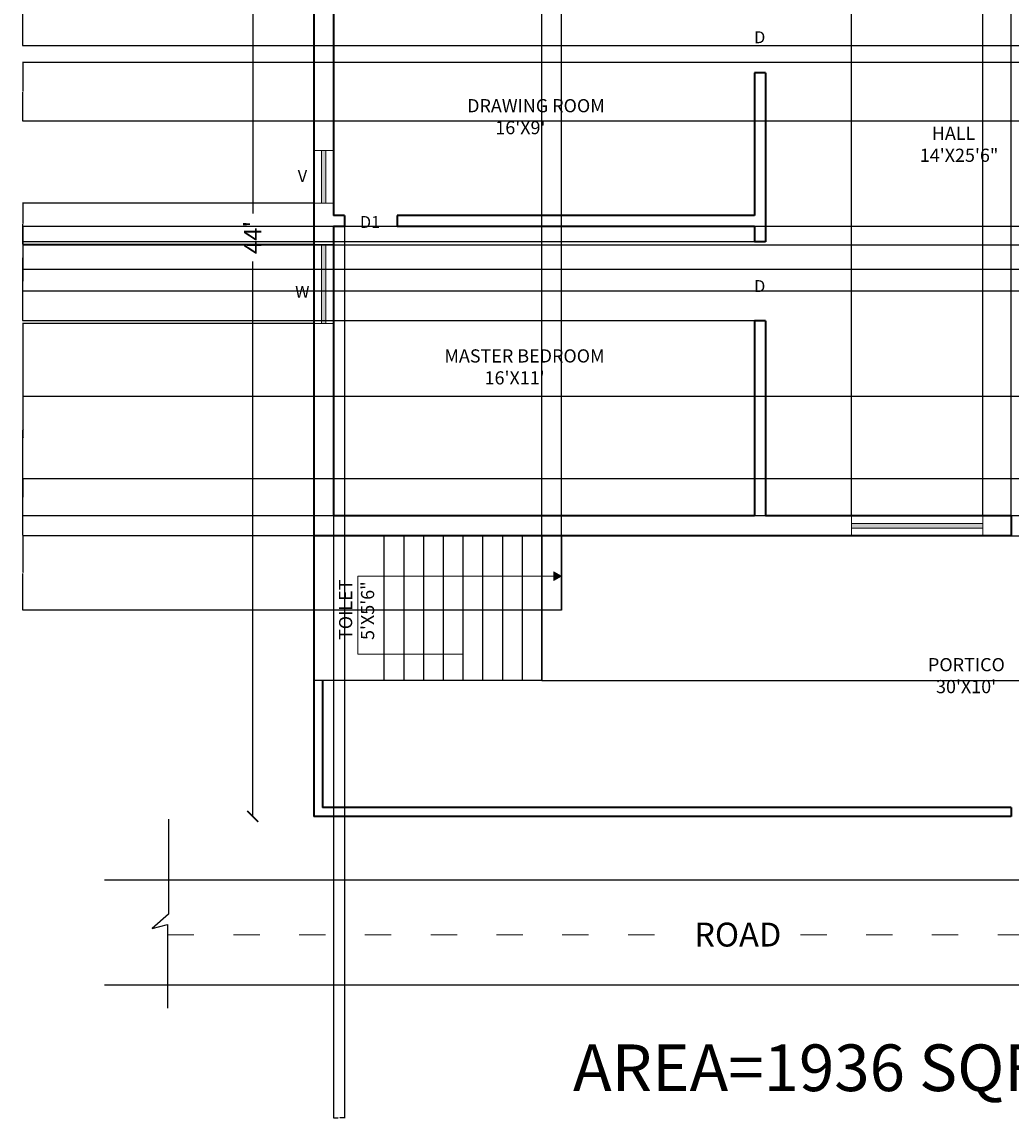
# Model space of a CAD drawing. Units: inches. Extents: x 320 to 1055, y -655 to 96.
# Tile 1 of 4: x 320 to 771, y -655 to -155. Entities that reach past the tile are written whole.
import ezdxf

# ---------------------------------------------------------------- set-up
doc = ezdxf.new("R2010")
doc.units = ezdxf.units.IN
doc.header["$MEASUREMENT"] = 0
doc.linetypes.add('ACAD_ISO03W100', pattern=[30, 12, -18])
for name, color, linetype, lineweight in [('A-ANNO-DIMS', 2, 'Continuous', 18), ('A-ANNO-IDEN', 1, 'Continuous', 18), ('A-ANNO-SYMB', 1, 'Continuous', 18), ('A-ANNO-TEXT', 8, 'Continuous', 18), ('A-AREA-IDEN', 8, 'Continuous', 18), ('A-FLOR-STRS', 1, 'Continuous', 25), ('A-GLAZ-PATT', 5, 'Continuous', 13), ('C-ROAD', 1, 'Continuous', 25), ('C-ROAD-CNTR', 1, 'ACAD_ISO03W100', 18), ('wall', 1, 'Continuous', 35), ('win', 5, 'Continuous', 18)]:
    doc.layers.add(name, color=color, linetype=linetype, lineweight=lineweight)
doc.styles.get("Standard").update_dxf_attribs({"font": 'arial.ttf'})
doc.dimstyles.get("Standard").update_dxf_attribs({"dimtxt": 0.18, "dimasz": 0.18, "dimexe": 0.18, "dimexo": 0.0625, "dimgap": 0.09, "dimtad": 0, "dimtih": 1, "dimtoh": 1, "dimdec": 1, "dimzin": 0, "dimdsep": 46, "dimlunit": 4, "dimtxsty": 'Standard', "dimcen": 0.09, "dimadec": 0, "dimazin": 0, "dimtfac": 1, "dimtdec": 1, "dimtofl": 0, "dimtmove": 0, "dimatfit": 3, "dimfxl": 1, "dimtolj": 1, "dimtzin": 0, "dimarcsym": 0})

# ---------------------------------------------------------------- blocks, each defined once
blk = doc.blocks.new('_ArchTick')
at = {"color": 0, "linetype": 'ByBlock', "const_width": 0.15}
blk.add_lwpolyline([(-0.5, -0.5), (0.5, 0.5)], dxfattribs=at)
blk = doc.blocks.new('*D2')
at = {"layer": 'A-ANNO-DIMS', "color": 0, "lineweight": -2, "transparency": 16777216}
for p, q in [((425, 10.26), (425, -242.79)), ((425, -517.74), (425, -264.69))]:
    blk.add_line(p, q, dxfattribs=at)
at = {"layer": 'Defpoints', "color": 0, "transparency": 16777216}
for p in [(452.86, 10.26), (425, -517.74), (452.86, -517.74)]:
    blk.add_point(p, dxfattribs=at)
at = {"layer": 'A-ANNO-DIMS', "color": 0, "lineweight": -2, "transparency": 16777216, "xscale": 5, "yscale": 5, "zscale": 5}
for p, rotation in [((425, 10.26), 90), ((425, -517.74), 270)]:
    blk.add_blockref('_ArchTick', p, dxfattribs=dict(at, rotation=rotation))
at = {"layer": 'A-ANNO-DIMS', "color": 0, "transparency": 16777216, "insert": (425, -253.74), "char_height": 8, "attachment_point": 5, "rotation": 90}
blk.add_mtext("\\A1;44'", dxfattribs=at)
blk = doc.blocks.new('WINDOW-36IN')
for p, q in [((0, 36), (9, 36)), ((3.5, 36), (3.5, 0)), ((5.5, 36), (5.5, 0)), ((0, 0), (9, 0))]:
    blk.add_line(p, q)
blk = doc.blocks.new('VENT-24IN')
for p, q in [((0, 0), (0, 9)), ((0, 5.5), (24, 5.5)), ((24, 0), (24, 9)), ((0, 3.5), (24, 3.5))]:
    blk.add_line(p, q)
blk = doc.blocks.new('*D21')
at = {"layer": 'A-ANNO-DIMS', "color": 0, "lineweight": -2, "transparency": 16777216}
for p, q in [((698.05, -380.67), (698.05, 47.57)), ((698.23, 47.39), (727.72, 47.39)), ((757.87, 47.39), (728.38, 47.39)), ((758.05, -380.67), (758.05, 47.57))]:
    blk.add_line(p, q, dxfattribs=at)
at = {"layer": 'A-ANNO-DIMS', "color": 0, "transparency": 16777216}
for points in [[(698.23, 47.42), (698.23, 47.36), (698.05, 47.39)], [(757.87, 47.42), (757.87, 47.36), (758.05, 47.39)]]:
    blk.add_solid(points, dxfattribs=at)
at = {"layer": 'Defpoints', "color": 0, "transparency": 16777216}
for p in [(758.05, 47.39), (698.05, -380.74), (758.05, -380.74)]:
    blk.add_point(p, dxfattribs=at)
at = {"layer": 'A-ANNO-DIMS', "color": 0, "transparency": 16777216, "insert": (728.05, 47.39), "char_height": 0.18, "attachment_point": 5}
blk.add_mtext('\\A1;5\'-0"', dxfattribs=at)
blk = doc.blocks.new('*D22')
at = {"layer": 'A-ANNO-DIMS', "color": 0, "lineweight": -2, "transparency": 16777216}
for p, q in [((658.8, -255.74), (320.04, -255.74)), ((320.22, -255.92), (320.22, -273.55)), ((320.22, -291.56), (320.22, -273.92)), ((658.8, -291.74), (320.04, -291.74))]:
    blk.add_line(p, q, dxfattribs=at)
at = {"layer": 'A-ANNO-DIMS', "color": 0, "transparency": 16777216}
for points in [[(320.19, -255.92), (320.25, -255.92), (320.22, -255.74)], [(320.19, -291.56), (320.25, -291.56), (320.22, -291.74)]]:
    blk.add_solid(points, dxfattribs=at)
at = {"layer": 'Defpoints', "color": 0, "transparency": 16777216}
for p in [(658.86, -255.74), (320.22, -291.74), (658.86, -291.74)]:
    blk.add_point(p, dxfattribs=at)
at = {"layer": 'A-ANNO-DIMS', "color": 0, "transparency": 16777216, "insert": (320.22, -273.74), "char_height": 0.18, "attachment_point": 5}
blk.add_mtext('\\A1;3\'-0"', dxfattribs=at)
blk = doc.blocks.new('*D26')
at = {"layer": 'A-ANNO-DIMS', "color": 0, "lineweight": -2, "transparency": 16777216}
for p, q in [((941.8, -248.74), (320.04, -248.74)), ((320.22, -248.92), (320.22, -263.27)), ((320.22, -278), (320.22, -263.64)), ((941.8, -278.18), (320.04, -278.18))]:
    blk.add_line(p, q, dxfattribs=at)
at = {"layer": 'A-ANNO-DIMS', "color": 0, "transparency": 16777216}
for points in [[(320.19, -248.92), (320.25, -248.92), (320.22, -248.74)], [(320.19, -278), (320.25, -278), (320.22, -278.18)]]:
    blk.add_solid(points, dxfattribs=at)
at = {"layer": 'Defpoints', "color": 0, "transparency": 16777216}
for p in [(941.86, -248.74), (320.22, -278.18), (941.86, -278.18)]:
    blk.add_point(p, dxfattribs=at)
at = {"layer": 'A-ANNO-DIMS', "color": 0, "transparency": 16777216, "insert": (320.22, -263.46), "char_height": 0.18, "attachment_point": 5}
blk.add_mtext('\\A1;2\'-5 1/2"', dxfattribs=at)
blk = doc.blocks.new('*D27')
at = {"layer": 'A-ANNO-DIMS', "color": 0, "lineweight": -2, "transparency": 16777216}
for p, q in [((943.8, -326.24), (320.04, -326.24)), ((320.22, -326.42), (320.22, -344.83)), ((320.22, -363.61), (320.22, -345.2)), ((943.8, -363.79), (320.04, -363.79))]:
    blk.add_line(p, q, dxfattribs=at)
at = {"layer": 'A-ANNO-DIMS', "color": 0, "transparency": 16777216}
for points in [[(320.19, -326.42), (320.25, -326.42), (320.22, -326.24)], [(320.19, -363.61), (320.25, -363.61), (320.22, -363.79)]]:
    blk.add_solid(points, dxfattribs=at)
at = {"layer": 'Defpoints', "color": 0, "transparency": 16777216}
for p in [(943.86, -326.24), (320.22, -363.79), (943.86, -363.79)]:
    blk.add_point(p, dxfattribs=at)
at = {"layer": 'A-ANNO-DIMS', "color": 0, "transparency": 16777216, "insert": (320.22, -345.02), "char_height": 0.18, "attachment_point": 5}
blk.add_mtext('\\A1;3\'-1 1/2"', dxfattribs=at)
blk = doc.blocks.new('*D32')
at = {"layer": 'A-ANNO-DIMS', "color": 0, "lineweight": -2, "transparency": 16777216}
for p, q in [((883.46, -174.02), (320.04, -174.02)), ((320.22, -174.2), (320.22, -187.17)), ((320.22, -200.52), (320.22, -187.54)), ((883.46, -200.7), (320.04, -200.7))]:
    blk.add_line(p, q, dxfattribs=at)
at = {"layer": 'A-ANNO-DIMS', "color": 0, "transparency": 16777216}
for points in [[(320.19, -174.2), (320.25, -174.2), (320.22, -174.02)], [(320.19, -200.52), (320.25, -200.52), (320.22, -200.7)]]:
    blk.add_solid(points, dxfattribs=at)
at = {"layer": 'Defpoints', "color": 0, "transparency": 16777216}
for p in [(883.52, -174.02), (320.22, -200.7), (883.52, -200.7)]:
    blk.add_point(p, dxfattribs=at)
at = {"layer": 'A-ANNO-DIMS', "color": 0, "transparency": 16777216, "insert": (320.22, -187.36), "char_height": 0.18, "attachment_point": 5}
blk.add_mtext('\\A1;2\'-2 1/2"', dxfattribs=at)
blk = doc.blocks.new('*D33')
at = {"layer": 'A-ANNO-DIMS', "color": 0, "lineweight": -2, "transparency": 16777216}
for p, q in [((452.86, -389.67), (452.86, 47.57)), ((453.04, 47.39), (509.03, 47.39)), ((565.68, 47.39), (509.69, 47.39)), ((565.86, -389.67), (565.86, 47.57))]:
    blk.add_line(p, q, dxfattribs=at)
at = {"layer": 'A-ANNO-DIMS', "color": 0, "transparency": 16777216}
for points in [[(453.04, 47.42), (453.04, 47.36), (452.86, 47.39)], [(565.68, 47.42), (565.68, 47.36), (565.86, 47.39)]]:
    blk.add_solid(points, dxfattribs=at)
at = {"layer": 'Defpoints', "color": 0, "transparency": 16777216}
for p in [(565.86, 47.39), (452.86, -389.74), (565.86, -389.74)]:
    blk.add_point(p, dxfattribs=at)
at = {"layer": 'A-ANNO-DIMS', "color": 0, "transparency": 16777216, "insert": (509.36, 47.39), "char_height": 0.18, "attachment_point": 5}
blk.add_mtext('\\A1;9\'-5"', dxfattribs=at)
blk = doc.blocks.new('*D34')
at = {"layer": 'A-ANNO-DIMS', "color": 0, "lineweight": -2, "transparency": 16777216}
for p, q in [((556.92, -389.74), (1054.75, -389.74)), ((1054.57, -389.92), (1054.57, -422.55)), ((1054.57, -455.56), (1054.57, -422.92)), ((556.92, -455.74), (1054.75, -455.74))]:
    blk.add_line(p, q, dxfattribs=at)
at = {"layer": 'A-ANNO-DIMS', "color": 0, "transparency": 16777216}
for points in [[(1054.54, -389.92), (1054.6, -389.92), (1054.57, -389.74)], [(1054.54, -455.56), (1054.6, -455.56), (1054.57, -455.74)]]:
    blk.add_solid(points, dxfattribs=at)
at = {"layer": 'Defpoints', "color": 0, "transparency": 16777216}
for p in [(556.86, -389.74), (556.86, -455.74), (1054.57, -455.74)]:
    blk.add_point(p, dxfattribs=at)
at = {"layer": 'A-ANNO-DIMS', "color": 0, "transparency": 16777216, "insert": (1054.57, -422.74), "char_height": 0.18, "attachment_point": 5}
blk.add_mtext('\\A1;5\'-6"', dxfattribs=at)
blk = doc.blocks.new('*D39')
at = {"layer": 'A-ANNO-DIMS', "color": 0, "lineweight": -2, "transparency": 16777216}
for p, q in [((452.8, -293.01), (320.04, -293.01)), ((320.22, -293.19), (320.22, -341.19)), ((320.22, -389.56), (320.22, -341.56)), ((452.8, -389.74), (320.04, -389.74))]:
    blk.add_line(p, q, dxfattribs=at)
at = {"layer": 'A-ANNO-DIMS', "color": 0, "transparency": 16777216}
for points in [[(320.19, -293.19), (320.25, -293.19), (320.22, -293.01)], [(320.19, -389.56), (320.25, -389.56), (320.22, -389.74)]]:
    blk.add_solid(points, dxfattribs=at)
at = {"layer": 'Defpoints', "color": 0, "transparency": 16777216}
for p in [(320.22, -293.01), (452.86, -293.01), (452.86, -389.74)]:
    blk.add_point(p, dxfattribs=at)
at = {"layer": 'A-ANNO-DIMS', "color": 0, "transparency": 16777216, "insert": (320.22, -341.37), "char_height": 0.18, "attachment_point": 5}
blk.add_mtext('\\A1;8\'-0 1/2"', dxfattribs=at)
blk = doc.blocks.new('*D41')
at = {"layer": 'A-ANNO-DIMS', "color": 0, "lineweight": -2, "transparency": 16777216}
for p, q in [((971.8, -135.74), (320.04, -135.74)), ((320.22, -135.92), (320.22, -150.86)), ((320.22, -166.18), (320.22, -151.23)), ((971.8, -166.36), (320.04, -166.36))]:
    blk.add_line(p, q, dxfattribs=at)
at = {"layer": 'A-ANNO-DIMS', "color": 0, "transparency": 16777216}
for points in [[(320.19, -135.92), (320.25, -135.92), (320.22, -135.74)], [(320.19, -166.18), (320.25, -166.18), (320.22, -166.36)]]:
    blk.add_solid(points, dxfattribs=at)
at = {"layer": 'Defpoints', "color": 0, "transparency": 16777216}
for p in [(971.86, -135.74), (320.22, -166.36), (971.86, -166.36)]:
    blk.add_point(p, dxfattribs=at)
at = {"layer": 'A-ANNO-DIMS', "color": 0, "transparency": 16777216, "insert": (320.22, -151.05), "char_height": 0.18, "attachment_point": 5}
blk.add_mtext('\\A1;2\'-6 1/2"', dxfattribs=at)
blk = doc.blocks.new('*D43')
at = {"layer": 'A-ANNO-DIMS', "color": 0, "lineweight": -2, "transparency": 16777216}
for p, q in [((943.8, -363.79), (320.04, -363.79)), ((320.22, -363.97), (320.22, -372.08)), ((320.22, -380.56), (320.22, -372.45)), ((941.8, -380.74), (320.04, -380.74))]:
    blk.add_line(p, q, dxfattribs=at)
at = {"layer": 'A-ANNO-DIMS', "color": 0, "transparency": 16777216}
for points in [[(320.19, -363.97), (320.25, -363.97), (320.22, -363.79)], [(320.19, -380.56), (320.25, -380.56), (320.22, -380.74)]]:
    blk.add_solid(points, dxfattribs=at)
at = {"layer": 'Defpoints', "color": 0, "transparency": 16777216}
for p in [(320.22, -363.79), (943.86, -363.79), (941.86, -380.74)]:
    blk.add_point(p, dxfattribs=at)
at = {"layer": 'A-ANNO-DIMS', "color": 0, "transparency": 16777216, "insert": (320.22, -372.26), "char_height": 0.18, "attachment_point": 5}
blk.add_mtext('\\A1;1\'-5"', dxfattribs=at)
blk = doc.blocks.new('*D44')
at = {"layer": 'A-ANNO-DIMS', "color": 0, "lineweight": -2, "transparency": 16777216}
for p, q in [((949.47, -257.26), (320.04, -257.26)), ((320.22, -257.44), (320.22, -262.61)), ((320.22, -268.14), (320.22, -262.97)), ((949.47, -268.32), (320.04, -268.32))]:
    blk.add_line(p, q, dxfattribs=at)
at = {"layer": 'A-ANNO-DIMS', "color": 0, "transparency": 16777216}
for points in [[(320.19, -257.44), (320.25, -257.44), (320.22, -257.26)], [(320.19, -268.14), (320.25, -268.14), (320.22, -268.32)]]:
    blk.add_solid(points, dxfattribs=at)
at = {"layer": 'Defpoints', "color": 0, "transparency": 16777216}
for p in [(949.54, -257.26), (320.22, -268.32), (949.54, -268.32)]:
    blk.add_point(p, dxfattribs=at)
at = {"layer": 'A-ANNO-DIMS', "color": 0, "transparency": 16777216, "insert": (320.22, -262.79), "char_height": 0.18, "attachment_point": 5}
blk.add_mtext('\\A1;0\'-11"', dxfattribs=at)
blk = doc.blocks.new('*D45')
at = {"layer": 'A-ANNO-DIMS', "color": 0, "lineweight": -2, "transparency": 16777216}
for p, q in [((452.8, -238.05), (320.04, -238.05)), ((320.22, -238.23), (320.22, -247.35)), ((320.22, -256.83), (320.22, -247.71)), ((452.8, -257.01), (320.04, -257.01))]:
    blk.add_line(p, q, dxfattribs=at)
at = {"layer": 'A-ANNO-DIMS', "color": 0, "transparency": 16777216}
for points in [[(320.19, -238.23), (320.25, -238.23), (320.22, -238.05)], [(320.19, -256.83), (320.25, -256.83), (320.22, -257.01)]]:
    blk.add_solid(points, dxfattribs=at)
at = {"layer": 'Defpoints', "color": 0, "transparency": 16777216}
for p in [(320.22, -238.05), (452.86, -238.05), (452.86, -257.01)]:
    blk.add_point(p, dxfattribs=at)
at = {"layer": 'A-ANNO-DIMS', "color": 0, "transparency": 16777216, "insert": (320.22, -247.53), "char_height": 0.18, "attachment_point": 5}
blk.add_mtext('\\A1;1\'-7"', dxfattribs=at)
blk = doc.blocks.new('*D46')
at = {"layer": 'A-ANNO-DIMS', "color": 0, "lineweight": -2, "transparency": 16777216}
for p, q in [((758.05, -380.67), (758.05, 47.57)), ((758.23, 47.39), (764.13, 47.39)), ((770.68, 47.39), (764.77, 47.39)), ((770.86, -380.67), (770.86, 47.57))]:
    blk.add_line(p, q, dxfattribs=at)
at = {"layer": 'A-ANNO-DIMS', "color": 0, "transparency": 16777216}
for points in [[(758.23, 47.42), (758.23, 47.36), (758.05, 47.39)], [(770.68, 47.42), (770.68, 47.36), (770.86, 47.39)]]:
    blk.add_solid(points, dxfattribs=at)
at = {"layer": 'Defpoints', "color": 0, "transparency": 16777216}
for p in [(770.86, 47.39), (758.05, -380.74), (770.86, -380.74)]:
    blk.add_point(p, dxfattribs=at)
at = {"layer": 'A-ANNO-DIMS', "color": 0, "transparency": 16777216, "insert": (764.45, 47.39), "char_height": 0.18, "attachment_point": 5}
blk.add_mtext('\\A1;1\'-1"', dxfattribs=at)
blk = doc.blocks.new('*D47')
at = {"layer": 'A-ANNO-DIMS', "color": 0, "lineweight": -2, "transparency": 16777216}
for p, q in [((653.8, -248.74), (320.04, -248.74)), ((320.22, -248.92), (320.22, -252.05)), ((320.22, -255.56), (320.22, -252.42)), ((653.8, -255.74), (320.04, -255.74))]:
    blk.add_line(p, q, dxfattribs=at)
at = {"layer": 'A-ANNO-DIMS', "color": 0, "transparency": 16777216}
for points in [[(320.19, -248.92), (320.25, -248.92), (320.22, -248.74)], [(320.19, -255.56), (320.25, -255.56), (320.22, -255.74)]]:
    blk.add_solid(points, dxfattribs=at)
at = {"layer": 'Defpoints', "color": 0, "transparency": 16777216}
for p in [(653.86, -248.74), (320.22, -255.74), (653.86, -255.74)]:
    blk.add_point(p, dxfattribs=at)
at = {"layer": 'A-ANNO-DIMS', "color": 0, "transparency": 16777216, "insert": (320.22, -252.24), "char_height": 0.18, "attachment_point": 5}
blk.add_mtext('\\A1;0\'-7"', dxfattribs=at)
blk = doc.blocks.new('*D48')
at = {"layer": 'A-ANNO-DIMS', "color": 0, "lineweight": -2, "transparency": 16777216}
for p, q in [((461.86, -248.8), (461.86, -655.29)), ((466.86, -248.8), (466.86, -655.29)), ((462.04, -655.11), (464.03, -655.11)), ((466.68, -655.11), (464.69, -655.11))]:
    blk.add_line(p, q, dxfattribs=at)
at = {"layer": 'A-ANNO-DIMS', "color": 0, "transparency": 16777216}
for points in [[(462.04, -655.08), (462.04, -655.14), (461.86, -655.11)], [(466.68, -655.08), (466.68, -655.14), (466.86, -655.11)]]:
    blk.add_solid(points, dxfattribs=at)
at = {"layer": 'Defpoints', "color": 0, "transparency": 16777216}
for p in [(461.86, -248.74), (466.86, -248.74), (466.86, -655.11)]:
    blk.add_point(p, dxfattribs=at)
at = {"layer": 'A-ANNO-DIMS', "color": 0, "transparency": 16777216, "insert": (464.36, -655.11), "char_height": 0.18, "attachment_point": 5}
blk.add_mtext('\\A1;0\'-5"', dxfattribs=at)
blk = doc.blocks.new('*D52')
at = {"layer": 'A-ANNO-DIMS', "color": 0, "lineweight": -2, "transparency": 16777216}
for p, q in [((556.86, -455.67), (556.86, 47.57)), ((557.04, 47.39), (561.03, 47.39)), ((565.68, 47.39), (561.69, 47.39)), ((565.86, -423.67), (565.86, 47.57))]:
    blk.add_line(p, q, dxfattribs=at)
at = {"layer": 'A-ANNO-DIMS', "color": 0, "transparency": 16777216}
for points in [[(557.04, 47.42), (557.04, 47.36), (556.86, 47.39)], [(565.68, 47.42), (565.68, 47.36), (565.86, 47.39)]]:
    blk.add_solid(points, dxfattribs=at)
at = {"layer": 'Defpoints', "color": 0, "transparency": 16777216}
for p in [(565.86, 47.39), (565.86, -423.74), (556.86, -455.74)]:
    blk.add_point(p, dxfattribs=at)
at = {"layer": 'A-ANNO-DIMS', "color": 0, "transparency": 16777216, "insert": (561.36, 47.39), "char_height": 0.18, "attachment_point": 5}
blk.add_mtext('\\A1;0\'-9"', dxfattribs=at)
blk = doc.blocks.new('*D53')
at = {"layer": 'A-ANNO-DIMS', "color": 0, "lineweight": -2, "transparency": 16777216}
for p, q in [((565.8, -389.74), (320.04, -389.74)), ((320.22, -389.92), (320.22, -406.55)), ((320.22, -423.56), (320.22, -406.92)), ((565.8, -423.74), (320.04, -423.74))]:
    blk.add_line(p, q, dxfattribs=at)
at = {"layer": 'A-ANNO-DIMS', "color": 0, "transparency": 16777216}
for points in [[(320.19, -389.92), (320.25, -389.92), (320.22, -389.74)], [(320.19, -423.56), (320.25, -423.56), (320.22, -423.74)]]:
    blk.add_solid(points, dxfattribs=at)
at = {"layer": 'Defpoints', "color": 0, "transparency": 16777216}
for p in [(320.22, -389.74), (565.86, -389.74), (565.86, -423.74)]:
    blk.add_point(p, dxfattribs=at)
at = {"layer": 'A-ANNO-DIMS', "color": 0, "transparency": 16777216, "insert": (320.22, -406.74), "char_height": 0.18, "attachment_point": 5}
blk.add_mtext('\\A1;2\'-10"', dxfattribs=at)

msp = doc.modelspace()

# ---------------------------------------------------------------- hatches: boundary and pattern name
at = {"layer": 'A-ANNO-SYMB'}
h = msp.add_hatch(color=256, dxfattribs=at)
h.dxf.hatch_style = 1
h.paths.add_polyline_path([(565.86, -408.22), (562.37, -406.22), (562.37, -408.22), (562.37, -410.22)])
at = {"layer": 'A-GLAZ-PATT'}
h = msp.add_hatch(color=256, dxfattribs=at)
h.dxf.hatch_style = 1
h.paths.add_polyline_path([(977.36, -166.36), (975.36, -166.36), (975.36, -214.36), (977.36, -214.36)])
h.paths.add_polyline_path([(977.36, -85.01), (975.36, -85.01), (975.36, -121.01), (977.36, -121.01)])
h.paths.add_polyline_path([(818.66, 6.76), (794.66, 6.76), (794.66, 4.76), (818.66, 4.76)])
h.paths.add_polyline_path([(689.3, 6.76), (665.3, 6.76), (665.3, 4.76), (689.3, 4.76)])
h.paths.add_polyline_path([(458.36, -10.79), (456.36, -10.79), (456.36, -46.79), (458.36, -46.79)])
h.paths.add_polyline_path([(458.36, -214.05), (456.36, -214.05), (456.36, -238.05), (458.36, -238.05)])
h.paths.add_polyline_path([(458.36, -257.01), (456.36, -257.01), (456.36, -293.01), (458.36, -293.01)])
h.paths.add_polyline_path([(977.36, -259), (975.36, -259), (975.36, -295), (977.36, -295)])
h.paths.add_polyline_path([(758.05, -384.24), (698.05, -384.24), (698.05, -386.24), (758.05, -386.24)])

# ---------------------------------------------------------------- linework, layer by layer
at = {"layer": 'A-ANNO-SYMB'}
for p, q in [((472.94, -443.75), (472.94, -408.22)), ((472.94, -408.22), (562.37, -408.22)), ((562.37, -408.22), (562.37, -406.22)), ((562.37, -406.22), (565.86, -408.22)), ((562.37, -408.22), (562.37, -410.22)), ((562.37, -410.22), (565.86, -408.22)), ((520.86, -443.75), (472.94, -443.75))]:
    msp.add_line(p, q, dxfattribs=at)
at = {"layer": 'A-FLOR-STRS'}
for p, q in [((484.86, -389.74), (484.86, -455.74)), ((493.86, -389.74), (493.86, -455.74)), ((502.86, -389.74), (502.86, -455.74)), ((511.86, -389.74), (511.86, -455.74)), ((520.86, -389.74), (520.86, -455.74)), ((529.86, -389.74), (529.86, -455.74)), ((538.86, -389.74), (538.86, -455.74)), ((547.86, -389.74), (547.86, -455.74)), ((556.86, -389.74), (556.86, -455.74)), ((565.86, -389.74), (565.86, -423.74)), ((565.86, -423.74), (484.86, -423.74)), ((556.86, -455.74), (452.86, -455.74))]:
    msp.add_line(p, q, dxfattribs=at)
at = {"layer": 'C-ROAD'}
for p, q in [((386.55, -519.06), (386.55, -562.36)), ((357.35, -546.58), (1017.02, -546.58)), ((386.55, -562.36), (379.08, -568.92)), ((379.08, -568.92), (386.2, -567.08)), ((386.2, -567.08), (386.2, -605.12)), ((357.35, -594.58), (1017.44, -594.58))]:
    msp.add_line(p, q, dxfattribs=at)
at = {"layer": 'C-ROAD-CNTR'}
for p, q in [((386.2, -571.77), (622.73, -571.77)), ((674.79, -571.77), (976.72, -571.77))]:
    msp.add_line(p, q, dxfattribs=at)
at = {"layer": 'wall'}
for p, q in [((452.86, 10.26), (452.86, -517.74)), ((452.86, 10.26), (452.86, -517.74)), ((461.86, -135.74), (461.86, -243.74)), ((658.86, -178.74), (653.86, -178.74)), ((653.86, -178.74), (653.86, -243.74)), ((658.86, -178.74), (658.86, -255.74)), ((466.86, -243.74), (461.86, -243.74)), ((466.86, -243.74), (466.86, -248.74)), ((653.86, -243.74), (490.86, -243.74)), ((490.86, -243.74), (490.86, -248.74)), ((461.86, -248.74), (461.86, -380.74)), ((466.86, -248.74), (461.86, -248.74)), ((653.86, -248.74), (490.86, -248.74)), ((653.86, -248.74), (653.86, -255.74)), ((658.86, -255.74), (653.86, -255.74)), ((658.86, -291.74), (653.86, -291.74)), ((653.86, -291.74), (653.86, -380.74)), ((658.86, -291.74), (658.86, -380.74)), ((653.86, -380.74), (461.86, -380.74)), ((770.86, -380.74), (658.86, -380.74)), ((770.86, -380.74), (770.86, -389.74)), ((770.86, -389.74), (452.86, -389.74)), ((456.86, -455.74), (456.86, -513.74)), ((770.86, -513.74), (456.86, -513.74)), ((770.86, -513.74), (770.86, -517.74)), ((770.86, -517.74), (452.86, -517.74)), ((770.86, -517.74), (452.86, -517.74))]:
    msp.add_line(p, q, dxfattribs=at)
at = {"layer": 'win'}
for p, q in [((698.05, -389.74), (698.05, -380.74)), ((758.05, -384.24), (698.05, -384.24)), ((758.05, -389.74), (758.05, -380.74)), ((758.05, -386.24), (698.05, -386.24))]:
    msp.add_line(p, q, dxfattribs=at)

# ---------------------------------------------------------------- block references
for name, p, rotation in [('VENT-24IN', (461.86, -238.05), 89.99999999999976), ('WINDOW-36IN', (461.86, -257.01), 180)]:
    msp.add_blockref(name, p, dxfattribs=dict(at, rotation=rotation))

# ---------------------------------------------------------------- texts
at = {"layer": 'A-ANNO-IDEN'}
for s, height, p in [('D', 5.44, (653.68, -165.17)), ('V', 5.44, (445.55, -228.45)), ('D1', 5.444, (473.9, -249.41)), ('D', 5.44, (653.68, -278.64)), ('W', 5.44, (444.36, -281.26))]:
    msp.add_text(s, height=height, dxfattribs=at).set_placement(p)
at = {"layer": 'A-ANNO-TEXT', "attachment_point": 1}
for s, width, gutter_width, insert, char_height in [('ROAD', 44.8037, 1.81, (626.36, -566.18), 10.889), ('AREA=1936 SQFT', 263.9184, 3.55, (571.05, -621.71), 21.2807)]:
    msp.add_mtext_dynamic_manual_height_columns(s, width=width, gutter_width=gutter_width, heights=[0], dxfattribs=dict(at, insert=insert, char_height=char_height))
at = {"layer": 'A-AREA-IDEN', "char_height": 6, "attachment_point": 1}
for s, width, insert in [("    DRAWING ROOM\\P           16'X9'", 81.9678, (515.47, -190.66)), ('         HALL\\P      14\'X25\'6"', 54.3765, (718.23, -203.26)), ("    MASTER BEDROOM\\P              16'X11'", 94.589, (505.08, -304.76)), ("   PORTICO\\P     30'X10'", 54.3765, (727.47, -445.54))]:
    msp.add_mtext_dynamic_manual_height_columns(s, width=width, gutter_width=1, heights=[0], dxfattribs=dict(at, insert=insert))
at = {"layer": 'A-AREA-IDEN', "insert": (464.38, -437.29), "char_height": 6, "attachment_point": 1, "rotation": 90}
msp.add_mtext_dynamic_manual_height_columns('TOILET      5\'X5\'6"', width=30.4605, gutter_width=1, heights=[0], dxfattribs=at)

# ---------------------------------------------------------------- dimensions: what is measured, and where the dimension line sits
at = {"layer": 'A-ANNO-DIMS'}
for base, p1, p2, picture, middle in [((565.86, 47.39), (452.86, -389.74), (565.86, -389.74), '*D33', (509.36, 47.39)), ((565.86, 47.39), (556.86, -455.74), (565.86, -423.74), '*D52', (561.36, 47.39)), ((758.05, 47.39), (698.05, -380.74), (758.05, -380.74), '*D21', (728.05, 47.39)), ((770.86, 47.39), (758.05, -380.74), (770.86, -380.74), '*D46', (764.45, 47.39)), ((466.86, -655.11), (461.86, -248.74), (466.86, -248.74), '*D48', (464.36, -655.11))]:
    dim = msp.add_linear_dim(base=base, p1=p1, p2=p2, dimstyle='Standard', override={"dimdec": 1, "dimlfac": 1, "dimrnd": 0, "dimzin": 1, "dimdsep": 46, "dimlunit": 4, "dimfrac": 2}, dxfattribs=at)
    dim.commit()
    dim.dimension.update_dxf_attribs({"geometry": picture, "text_midpoint": middle})
for base, p1, p2, override, picture, middle in [((425, -517.74), (452.86, 10.26), (452.86, -517.74), {"dimtxt": 8, "dimasz": 5, "dimgap": 4, "dimtih": 0, "dimblk1": 'ArchTick', "dimblk2": 'ArchTick', "dimsah": 1, "dimse1": 1, "dimse2": 1, "dimclrd": 0, "dimclre": 0, "dimclrt": 0}, '*D2', (425, -253.74)), ((320.22, -166.36), (971.86, -135.74), (971.86, -166.36), {"dimdec": 1, "dimlfac": 1, "dimrnd": 0, "dimzin": 1, "dimdsep": 46, "dimlunit": 4, "dimfrac": 2}, '*D41', (320.22, -151.05)), ((320.22, -200.7), (883.52, -174.02), (883.52, -200.7), {"dimdec": 1, "dimlfac": 1, "dimrnd": 0, "dimzin": 1, "dimdsep": 46, "dimlunit": 4, "dimfrac": 2}, '*D32', (320.22, -187.36)), ((320.22, -238.05), (452.86, -257.01), (452.86, -238.05), {"dimdec": 1, "dimlfac": 1, "dimrnd": 0, "dimzin": 1, "dimdsep": 46, "dimlunit": 4, "dimfrac": 2}, '*D45', (320.22, -247.53)), ((320.22, -278.18), (941.86, -248.74), (941.86, -278.18), {"dimdec": 1, "dimlfac": 1, "dimrnd": 0, "dimzin": 1, "dimdsep": 46, "dimlunit": 4, "dimfrac": 2}, '*D26', (320.22, -263.46)), ((320.22, -255.74), (653.86, -248.74), (653.86, -255.74), {"dimdec": 1, "dimlfac": 1, "dimrnd": 0, "dimzin": 1, "dimdsep": 46, "dimlunit": 4, "dimfrac": 2}, '*D47', (320.22, -252.24)), ((320.22, -268.32), (949.54, -257.26), (949.54, -268.32), {"dimdec": 1, "dimlfac": 1, "dimrnd": 0, "dimzin": 1, "dimdsep": 46, "dimlunit": 4, "dimfrac": 2}, '*D44', (320.22, -262.79)), ((320.22, -291.74), (658.86, -255.74), (658.86, -291.74), {"dimdec": 1, "dimlfac": 1, "dimrnd": 0, "dimzin": 1, "dimdsep": 46, "dimlunit": 4, "dimfrac": 2}, '*D22', (320.22, -273.74)), ((320.22, -293.01), (452.86, -389.74), (452.86, -293.01), {"dimdec": 1, "dimlfac": 1, "dimrnd": 0, "dimzin": 1, "dimdsep": 46, "dimlunit": 4, "dimfrac": 2}, '*D39', (320.22, -341.37)), ((320.2225, -363.7938), (943.8635, -326.2397), (943.8635, -363.7938), {"dimdec": 1, "dimlfac": 1, "dimrnd": 0, "dimzin": 1, "dimdsep": 46, "dimlunit": 4, "dimfrac": 2}, '*D27', (320.2225, -345.0167)), ((320.2225, -363.7938), (941.8589, -380.7361), (943.8635, -363.7938), {"dimdec": 1, "dimlfac": 1, "dimrnd": 0, "dimzin": 1, "dimdsep": 46, "dimlunit": 4, "dimfrac": 2}, '*D43', (320.2225, -372.265)), ((320.22, -389.74), (565.86, -423.74), (565.86, -389.74), {"dimdec": 1, "dimlfac": 1, "dimrnd": 0, "dimzin": 1, "dimdsep": 46, "dimlunit": 4, "dimfrac": 2}, '*D53', (320.22, -406.74)), ((1054.57, -455.74), (556.86, -389.74), (556.86, -455.74), {"dimdec": 1, "dimlfac": 1, "dimrnd": 0, "dimzin": 1, "dimdsep": 46, "dimlunit": 4, "dimfrac": 2}, '*D34', (1054.57, -422.74))]:
    dim = msp.add_linear_dim(base=base, p1=p1, p2=p2, angle=90, dimstyle='Standard', override=override, dxfattribs=at)
    dim.commit()
    dim.dimension.update_dxf_attribs({"geometry": picture, "text_midpoint": middle})

doc.saveas('drawing.dxf')
